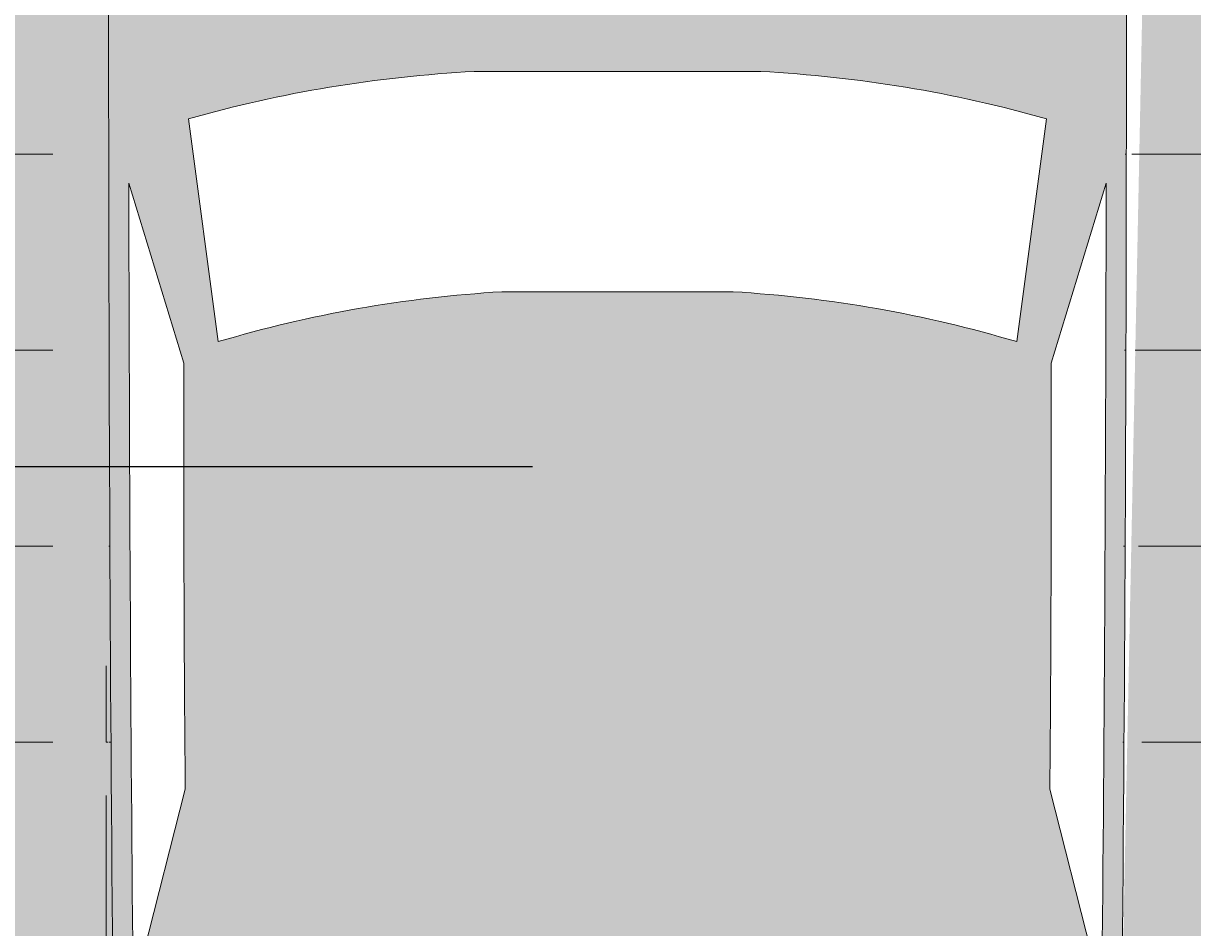
# Model space of a CAD drawing. Units: millimetres. Extents: x 1166 to 16630, y -7192 to 2820.
# Tile 4 of 8: x 5842 to 7051, y -4887 to -3952. Entities that reach past the tile are written whole.
import ezdxf

# ---------------------------------------------------------------- set-up
doc = ezdxf.new("R2010")
doc.units = ezdxf.units.MM
for name, color, linetype, lineweight in [('A-ANNO-DIMS', 2, 'Continuous', 18), ('A-FLOR-PATT', 8, 'Continuous', 13), ('C-PKNG-VEHI', 8, 'Continuous', 18)]:
    doc.layers.add(name, color=color, linetype=linetype, lineweight=lineweight)
doc.layers.add('A-FLOR-FNSH-PATT', color=254, linetype='Continuous', lineweight=13, true_color=0xfeeab9)
doc.layers.add('C-PKNG-VEHI-PATT', color=18, linetype='Continuous', lineweight=13, true_color=0x000000)
doc.styles.get("Standard").update_dxf_attribs({"font": 'arial.ttf'})
doc.dimstyles.get("Standard").update_dxf_attribs({"dimtxt": 0.18, "dimasz": 0.18, "dimexe": 0.18, "dimexo": 0.0625, "dimgap": 0.09, "dimtad": 0, "dimtih": 1, "dimtoh": 1, "dimdec": 4, "dimzin": 0, "dimdsep": 46, "dimtxsty": 'Standard', "dimcen": 0.09, "dimadec": 0, "dimazin": 0, "dimtfac": 1, "dimtdec": 4, "dimtofl": 0, "dimtmove": 0, "dimatfit": 3, "dimfxl": 1, "dimtolj": 1, "dimtzin": 0, "dimarcsym": 0})

# ---------------------------------------------------------------- blocks, each defined once
blk = doc.blocks.new('*U6')
for p, q in [((87.98532186932616, 31.87120872459877), (74.75900729854769, 35.92175679182955)), ((134.313356548143, 35.6043097713567), (119.2882629232503, 31.77757799177584)), ((70.0302824853563, 31.53613089391356), (86.40615155322342, 29.35124891408057)), ((66.55009204259746, -10.5288681329018), (66.55009204259746, 10.52886813290129)), ((82.73706193978568, 8.496039918672748), (82.73706193978568, -8.49603991867258)), ((86.40615155322318, -29.35124891408145), (70.03028248535594, -31.53613089391442)), ((134.3133565481428, -35.60430977135721), (119.2882629232503, -31.77757799177618)), ((87.98532186932607, -31.87120872459903), (74.7590072985476, -35.92175679182964))]:
    blk.add_line(p, q)
for centre, major_axis, ratio, start_param, end_param in [((64.48199294511879, -10555.61767587835), (1.907644e-10, 10593.02630634627), 0.842303869543847, -0.0133969486112073, 0.0027970409639888), ((64.4819929449925, -10555.61767590795), (1.9177683e-09, -10591.54646030096), 0.8423038695482963, 3.133765086725325, 3.140440689641252), ((95.78879860270445, -3666.353346297651), (1.949864e-10, -3698.236159209632), 0.8423038695446962, 3.134048706297306, 3.14409775411291), ((135.2911776514449, 5.387441675478555), (2.2715e-12, 81.77258453065997), 0.8423038695439563, 1.245306111696802, 1.507880129813836), ((149.595361812917, 2.799442537139299), (8.561e-13, -79.57966406425402), 0.842303869543983, 4.372215489277867, 4.640744122441986), ((149.5953618129329, -2.799442537137565), (4.0897e-12, -79.57966406427697), 0.8423038695439419, -1.499151468852248, -1.230622835688196), ((135.2911776514465, -5.387441675480715), (3.2038e-12, -81.77258453066244), 0.8423038695439492, -1.50788012981387, -1.245306111696839), ((95.78879860271888, 3666.35334629765), (1.637818e-10, -3698.236159209629), 0.8423038695447546, -0.0025051005232382, 0.007543947292366), ((64.48199294503607, 10555.61767590793), (1.6049794e-09, -10591.54646030094), 0.8423038695397146, 0.0011519639481523, 0.0078275668641468), ((64.48199294495228, 10555.61767590795), (6.117947e-10, 10593.02630637587), 0.8423038695458146, 3.138795612625926, 3.154989602201039)]:
    blk.add_ellipse(centre, major_axis=major_axis, ratio=ratio, start_param=start_param, end_param=end_param)
blk = doc.blocks.new('*D69')
at = {"layer": 'A-ANNO-DIMS', "color": 0, "lineweight": -2, "transparency": 16777216}
for p, q in [((2812.839545999997, -4410.708250999998), (2813.019545999998, -4410.708250999998)), ((2812.929545999998, -4410.798250999998), (2812.929545999998, -4410.618250999998)), ((6334.94458279999, -4410.707849399996), (5014.368944, -4410.707999979473))]:
    blk.add_line(p, q, dxfattribs=at)
at = {"layer": 'A-ANNO-DIMS', "color": 0, "transparency": 16777216}
blk.add_solid([(5014.36894399658, -4410.677999979474), (5014.368944003422, -4410.737999979473), (5014.188944, -4410.707999999998)], dxfattribs=at)
at = {"layer": 'Defpoints', "color": 0, "transparency": 16777216}
for p in [(2812.929545999998, -4410.708250999998), (5014.188944, -4410.707999999998)]:
    blk.add_point(p, dxfattribs=at)
at = {"layer": 'A-ANNO-DIMS', "color": 0, "transparency": 16777216, "insert": (6335.494344055106, -4410.707849399996), "char_height": 0.18, "attachment_point": 5}
blk.add_mtext('\\A1;R2201.3', dxfattribs=at)
blk = doc.blocks.new('*D70')
at = {"layer": 'A-ANNO-DIMS', "color": 0, "lineweight": -2, "transparency": 16777216}
for p, q in [((3047.988206, -4410.708432999997), (3048.168206000001, -4410.708432999997)), ((3048.078206, -4410.798432999997), (3048.078206, -4410.618432999997)), ((6368.217169199974, -4410.707740199998), (5123.345058, -4410.707999962437))]:
    blk.add_line(p, q, dxfattribs=at)
at = {"layer": 'A-ANNO-DIMS', "color": 0, "transparency": 16777216}
blk.add_solid([(5123.34505799374, -4410.677999962437), (5123.34505800626, -4410.737999962437), (5123.165058, -4410.707999999998)], dxfattribs=at)
at = {"layer": 'Defpoints', "color": 0, "transparency": 16777216}
for p in [(3048.078206, -4410.708432999998), (5123.165058, -4410.707999999998)]:
    blk.add_point(p, dxfattribs=at)
at = {"layer": 'A-ANNO-DIMS', "color": 0, "transparency": 16777216, "insert": (6368.662749008977, -4410.707740199998), "char_height": 0.18, "attachment_point": 5}
blk.add_mtext('\\A1;R2075', dxfattribs=at)

msp = doc.modelspace()

# ---------------------------------------------------------------- hatches: boundary and pattern name
at = {"layer": 'A-FLOR-FNSH-PATT', "transparency": 33554590}
h = msp.add_hatch(color=256, dxfattribs=at)
h.dxf.hatch_style = 1
h.paths.add_polyline_path([(5309.614992693758, -2642.53776490782), (5309.614992693758, -6304.141088113749), (7725.939441137629, -6304.141088113749), (7725.939441137629, -5672.53776490782), (7725.939441137629, -2642.53776490782)])
edge = h.paths.add_edge_path(flags=16)
edge.add_ellipse((-448.9724108440159, -3645.429588524165), major_axis=(-7430.722679011307, 2.05049e-10), ratio=0.8423038695440578, start_angle=182.1799503136468, end_angle=183.6504275857006, ccw=False)
edge.add_line((6974.17381326888, -3362.862478220109), (6984.715647929133, -3362.862478220109))
edge.add_ellipse((6982.28108362224, -3380.396843230207), major_axis=(-20.81714882728829, 5.19e-13), ratio=0.842303869543992, start_angle=180.0000000000014, end_angle=270.0000000000014, ccw=False)
edge.add_line((7003.098232449528, -3380.396843230198), (7003.098232449528, -3722.915565549822))
edge.add_ellipse((6982.28108362224, -3720.864922613471), major_axis=(20.81714882728829, 5.097e-13), ratio=0.842303869543992, start_angle=269.9999999999985, end_angle=359.9999999999986, ccw=False)
edge.add_ellipse((-142030.922985108, -3973.064272051784), major_axis=(149013.2040687302, 7.3876543e-09), ratio=0.8423038695454406, start_angle=-0.3838667787953227, end_angle=0.09022908859151357, ccw=False)
edge.add_line((6977.567346638728, -4971.397229994678), (6984.470063297348, -4971.397229994678))
edge.add_ellipse((6982.28108362224, -4988.931595004776), major_axis=(20.81714882728829, 5.4695e-12), ratio=0.84230386954397, start_angle=-1.5006662579253316e-11, end_angle=89.99999999998488, ccw=False)
edge.add_line((7003.098232449528, -4988.931595004766), (7003.098232449527, -5331.243460438734))
edge.add_ellipse((6982.281083622239, -5329.399674388036), major_axis=(-20.81714882728829, 1.0505e-12), ratio=0.84230386954397, start_angle=90.0000000000029, end_angle=180.000000000003, ccw=False)
edge.add_line((6982.281083622243, -5346.934039398132), (6973.353954790083, -5346.934039398132))
edge.add_ellipse((-142030.922985108, -3973.064272051784), major_axis=(149013.2040687302, 7.3876543e-09), ratio=0.8423038695454406, start_angle=-0.6186431963221253, end_angle=-0.5282714718208013, ccw=False)
edge.add_ellipse((6960.189207408767, -5606.902802775503), major_axis=(-31.22572324093233, 2.0889e-12), ratio=0.8423038695439425, start_angle=179.3717627838109, end_angle=248.4647566010108, ccw=False)
edge.add_ellipse((-142041.331559525, -3973.064272085929), major_axis=(-149045.3717863939, 4.64621177404e-05), ratio=0.8423038661083152, start_angle=179.3534459208122, end_angle=179.3717628016453, ccw=False)
edge.add_ellipse((6916.869834512962, -5654.054118847628), major_axis=(-73.80201542105252, 3.6097e-12), ratio=0.8423038695439748, start_angle=90.00000000006492, end_angle=179.353445902922, ccw=False)
edge.add_line((6916.869834513031, -5716.217842016925), (5995.230132669023, -5716.217842016909))
edge.add_ellipse((5995.230132669163, -5654.054118847574), major_axis=(73.80201542109666, 3.978e-13), ratio=0.8423038695439887, start_angle=180.6465540970575, end_angle=269.9999999998622, ccw=False)
edge.add_ellipse((154953.4315273228, -3973.06427200764), major_axis=(-149045.3717871212, 2.2898328512e-06), ratio=0.8423038697262194, start_angle=0.6282372171232851, end_angle=0.6465540979564253, ccw=False)
edge.add_ellipse((5951.910759773294, -5606.902802775455), major_axis=(31.22572324094488, 4.9039e-12), ratio=0.842303869543988, start_angle=111.53524350401449, end_angle=180.6282372161637, ccw=False)
edge.add_ellipse((154943.0229527065, -3973.064272049507), major_axis=(-149013.2040691466, 7.4869171e-09), ratio=0.8423038695459824, start_angle=0.528271471820176, end_angle=0.6465540970638131, ccw=False)
edge.add_line((5938.746012391977, -5346.934039398132), (5927.384319252956, -5346.934039398132))
edge.add_ellipse((5929.818883559845, -5329.399674388033), major_axis=(20.8171488272892, 3.11e-13), ratio=0.8423038695440205, start_angle=179.9999999999992, end_angle=269.9999999999962, ccw=False)
edge.add_line((5909.001734732555, -5329.399674388034), (5909.001734732554, -4986.88095206843))
edge.add_ellipse((5929.818883559843, -4988.931595004776), major_axis=(-20.8171488272892, 3.063e-13), ratio=0.8423038695440205, start_angle=-89.99999999999608, end_angle=7.958078640513122e-13, ccw=False)
edge.add_line((5929.818883559843, -4971.397229994676), (5934.53262054336, -4971.397229994676))
edge.add_ellipse((154943.0229527065, -3973.064272049507), major_axis=(-149013.2040691466, 7.4869171e-09), ratio=0.8423038695459824, start_angle=-0.09022908859031986, end_angle=0.38386677879520903, ccw=False)
edge.add_ellipse((5929.818883559843, -3720.864922613471), major_axis=(-20.8171488272892, 1.5867e-12), ratio=0.8423038695439331, start_angle=4.376943252282217e-12, end_angle=90.00000000000438, ccw=False)
edge.add_line((5909.001734732555, -3720.864922613478), (5909.001734732555, -3378.346200293855))
edge.add_ellipse((5929.818883559843, -3380.396843230207), major_axis=(20.8171488272892, 9.396e-13), ratio=0.8423038695439548, start_angle=89.99999999999739, end_angle=179.9999999999975, ccw=False)
edge.add_line((5929.818883559843, -3362.862478220109), (5937.926153913206, -3362.862478220109))
edge.add_ellipse((13361.0723780261, -3645.42958852417), major_axis=(7430.722679011307, 7.96527e-11), ratio=0.8423038695440075, start_angle=176.3495724143003, end_angle=177.8200496863542, ccw=False)
edge.add_ellipse((6843.238962592569, -6808.26137511002), major_axis=(4407.332901654202, 4.993684e-10), ratio=0.8423038695438785, start_angle=102.12596555227748, end_angle=103.7805289894913, ccw=False)
edge.add_ellipse((6843.238962592481, -6711.831352601092), major_axis=(4294.727564406183, 8.108409e-10), ratio=0.8423038695438188, start_angle=100.20953899713243, end_angle=102.4446272934332, ccw=False)
edge.add_ellipse((5718.978043047074, -189.3416182050969), major_axis=(-3530.283493235897, 2.29487e-11), ratio=0.8423038695439934, start_angle=99.25656600720184, end_angle=102.5549326441376)
edge.add_line((6369.842688727707, -3111.939026631001), (6452.046781461999, -3066.482546539763))
edge.add_ellipse((6456.049983591043, -3074.756545497792), major_axis=(-10.40857441364578, 1.5838e-12), ratio=0.8423038695437935, start_angle=270.0000000000206, end_angle=307.9331304598557, ccw=False)
edge.add_ellipse((6456.049983591043, -3074.756545497792), major_axis=(-10.40857441364578, 1.5838e-12), ratio=0.8423038695437935, start_angle=232.06686954016618, end_angle=270.0000000000206, ccw=False)
edge.add_line((6461.762224667734, -3067.427595530816), (6542.257278454378, -3111.939026631002))
edge.add_ellipse((7193.121924135012, -189.3416182050969), major_axis=(3530.283493235459, 5.426614e-10), ratio=0.842303869544094, start_angle=257.4450673558539, end_angle=260.7434339927895)
edge.add_ellipse((6068.861004589511, -6711.831352601148), major_axis=(4294.72756440461, 7.517164e-10), ratio=0.8423038695441345, start_angle=77.55537270654469, end_angle=79.79046100284552, ccw=False)
edge.add_ellipse((6068.86100458951, -6808.26137511002), major_axis=(-4407.332901654327, 6.637773e-10), ratio=0.842303869543856, start_angle=256.2194710105107, end_angle=257.8740344477245, ccw=False)
edge = h.paths.add_edge_path(flags=0)
edge.add_ellipse((5799.636342679871, -3484.80630294614), major_axis=(790.1331889300527, 2.1537e-12), ratio=0.8423038695439757, start_angle=-2.2737367544323206e-13, end_angle=29.43856959797921, ccw=False)
edge.add_line((6589.769531609924, -3484.806302946152), (6589.769531609924, -3517.865771969153))
edge.add_line((6589.769531609924, -3517.865771969153), (6615.396946753699, -3517.865771969153))
edge.add_ellipse((6612.950235160742, -3526.632954474201), major_axis=(10.40857441364348, 1.5653e-12), ratio=0.8423038695440233, start_angle=45.51978911742219, end_angle=89.99999999999147, ccw=False)
edge.add_line((6619.58436781158, -3519.877346340421), (6697.576744801804, -3574.216072032502))
edge.add_line((6697.576744801804, -3574.216072032502), (6697.576744801804, -3782.552340767745))
edge.add_ellipse((6643.673138205864, -3780.461483581003), major_axis=(5.016450041930374, 89.18653102701357), ratio=0.6038335755719256, start_angle=106.34259195429391, end_angle=270.99798572497, ccw=False)
edge.add_line((6589.769531609924, -3793.028339937766), (6589.769531609924, -3484.806302946153))
edge.add_ellipse((5799.636342679871, -3484.80630294614), major_axis=(790.1331889300527, 2.1537e-12), ratio=0.8423038695439757, start_angle=-2.143e-13, end_angle=29.43856959797918)
edge.add_ellipse((7112.463624502211, -3484.80630294614), major_axis=(-790.1331889300524, 7.9434e-12), ratio=0.8423038695439707, start_angle=-29.43856959797882, end_angle=5.465e-13)
edge.add_line((6322.330435572158, -3484.806302946151), (6322.330435572158, -3793.028339937766))
edge.add_ellipse((6268.426828976219, -3780.461483581003), major_axis=(-5.016450041930374, 89.18653102701357), ratio=0.6038335755719256, start_angle=89.00201427502998, end_angle=253.6574080457062, ccw=False)
edge.add_line((6214.523222380278, -3782.552340767737), (6214.523222380279, -3574.216072032502))
edge.add_line((6214.523222380279, -3574.216072032502), (6294.400928520307, -3518.563802793423))
edge.add_ellipse((6299.149732021341, -3526.632954474201), major_axis=(10.4085744136453, 3.381e-13), ratio=0.8423038695438764, start_angle=89.9999999999983, end_angle=134.4802108825654, ccw=False)
edge.add_line((6299.149732021338, -3517.865771969152), (6322.330435572158, -3517.865771969152))
edge.add_line((6322.330435572158, -3517.865771969152), (6322.330435572158, -3484.806302946154))
edge.add_ellipse((7112.463624502211, -3484.80630294614), major_axis=(-790.1331889300524, 7.9434e-12), ratio=0.8423038695439707, start_angle=-29.438569597978812, end_angle=6.252776074688882e-13, ccw=False)
edge = h.paths.add_edge_path(flags=0)
edge.add_line((6899.672020630411, -4051.112638739672), (6868.937058315451, -4281.473694083312))
edge.add_ellipse((6495.430033257824, -5170.362894493258), major_axis=(1119.455420763322, 3.0514e-12), ratio=0.8423038695439744, start_angle=67.20808512240981, end_angle=85.12993040286408)
edge.add_line((6575.564661792019, -4229.860228440724), (6336.53530539007, -4229.860228440724))
edge.add_ellipse((6416.669933924288, -5170.362894493482), major_axis=(1119.455420763633, 5.82337e-11), ratio=0.842303869543943, start_angle=94.87006959713275, end_angle=112.7919148775836)
edge.add_line((6043.162908866626, -4281.473694083309), (6012.427946551666, -4051.112638739666))
edge.add_ellipse((6380.264280565288, -4969.144446445703), major_axis=(1150.303461305961, 5.9583e-11), ratio=0.8423038695439412, start_angle=94.27742096305099, end_angle=111.83495379670521, ccw=False)
edge.add_line((6307.939299228742, -4002.156437400477), (6604.160667953341, -4002.156437400477))
edge.add_ellipse((6531.835686616772, -4969.144446445682), major_axis=(-1150.303461305901, 2.25473e-11), ratio=0.8423038695439672, start_angle=248.1650462032914, end_angle=265.72257903694555, ccw=False)
edge = h.paths.add_edge_path(flags=0)
edge.add_ellipse((-142030.9229855244, -3973.064272050007), major_axis=(-148992.3869203194, 2.076209e-10), ratio=0.842303869544003, start_angle=179.6222358060902, end_angle=179.9444056865007, ccw=False)
edge.add_line((6956.899516505626, -4955.389335168179), (6903.06848209712, -4744.029778632651))
edge.add_ellipse((-45118.92430422086, -4413.460367112857), major_axis=(52023.47313689829, 7.771381e-10), ratio=0.842303869543516, start_angle=-0.3640763488911976, end_angle=0.1208973690317991)
edge.add_line((6904.3855953652, -4303.688047353878), (6961.365076797346, -4117.63210307358))
edge = h.paths.add_edge_path(flags=0)
edge.add_line((5950.734890384741, -4117.632103073563), (6007.714371816899, -4303.688047353918))
edge.add_ellipse((58031.02427140294, -4413.460367113082), major_axis=(-52023.47313689826, 1.3200601e-09), ratio=0.8423038695497072, start_angle=-0.1208973690315197, end_angle=0.364076348891516)
edge.add_line((6009.031485084967, -4744.029778632643), (5955.200450676423, -4955.389335168309))
edge.add_ellipse((154943.0229527063, -3973.064272050686), major_axis=(-148992.3869203192, 3.28274152e-08), ratio=0.8423038695536886, start_angle=0.05559431351167632, end_angle=0.3777641939223031, ccw=False)
edge = h.paths.add_edge_path(flags=0)
edge.add_line((6868.937058315452, -5013.198477251068), (6868.937058315452, -5277.993200767081))
edge.add_ellipse((6456.049983591043, -3571.079447459644), major_axis=(2068.11644385622, 7.9333e-12), ratio=0.8423038695439821, start_angle=256.4018653097692, end_angle=283.59813469023027, ccw=False)
edge.add_line((6043.16290886663, -5277.993200767081), (6043.16290886663, -5013.198477251068))
edge.add_ellipse((6456.049983591043, -3306.284723943631), major_axis=(2068.116443856253, 3.3411e-12), ratio=0.8423038695439679, start_angle=256.4018653097692, end_angle=283.5981346902304)
edge = h.paths.add_edge_path(flags=0)
edge.add_ellipse((6827.302760660877, -5415.313265203762), major_axis=(-41.63429765457658, 1.038e-12), ratio=0.842303869543992, start_angle=180.0000000000014, end_angle=270.0000000000014, ccw=False)
edge.add_line((6868.937058315454, -5415.313265203762), (6868.937058315454, -5689.12284886784))
edge.add_line((6868.937058315454, -5689.12284886784), (6043.162908866631, -5689.122848867824))
edge.add_line((6043.162908866631, -5689.122848867824), (6043.16290886663, -5415.313265203758))
edge.add_ellipse((6084.797206521206, -5415.313265203759), major_axis=(-41.63429765457658, 3.4138e-12), ratio=0.842303869543992, start_angle=-89.99999999999523, end_angle=4.718003765447065e-12, ccw=False)
edge.add_line((6084.797206521207, -5380.244535183563), (6827.302760660879, -5380.244535183566))
h.paths.add_polyline_path([(3455.939441137629, -522.53776490782), (1955.939441137629, -522.53776490782), (1955.939441137629, -2522.53776490782), (3455.939441137629, -2522.53776490782), (3455.939441137628, -2456.640093510054), (2713.439441137629, -2456.640093510054), (2713.43944113763, -2423.827593510054), (2714.157558370035, -2423.827593510054, -0.398552660000795), (3455.939441137629, -1706.6775944476)])
h.paths.add_polyline_path([(2617.666699633915, -1084.404517764245, -0.1328909081885223), (2584.2707950462, -1084.404517500826, -0.5013167773008519), (2505.064916213601, -782.9330743979599), (2537.033121160981, -687.0284595558127), (2489.081652205778, -687.0284595558132), (2489.081652205778, -711.0041940334158), (2441.130183250573, -711.0041940334158), (2441.130183250573, -695.0203710483474), (2473.097829220709, -695.0203710483474), (2473.097829220709, -687.0284595558132), (2433.13827175804, -687.0284595558132), (2433.138271758038, -559.1578756752674), (2768.79855444447, -559.1578756752674), (2768.798554444471, -687.0284595558132), (2664.903705041528, -687.0284595558132), (2696.870765296628, -782.9296403211174, -0.5013234908365807)], flags=16)
h.paths.add_polyline_path([(2627.246667254758, -1063.015793855155, -0.2150037826753064), (2574.690827957319, -1063.015793301825, -0.4800796505537303), (2537.033991046725, -782.9313974662227), (2664.904416594217, -782.9313974662227, -0.4800795019660876)], flags=0)
h.paths.add_polyline_path([(2736.830905816404, -671.0446365707452), (2465.105920386107, -671.0446365707452, -0.5000001164022092), (2449.122094743107, -655.0608109277463), (2449.122094743107, -591.1255243033341, -0.5000001164022404), (2465.105920386111, -575.1416986603361), (2736.830905816402, -575.1416986603361, -0.5000001164023353), (2752.814731459403, -591.1255243033406), (2752.814731459403, -655.0608109277468, -0.50000011640211)], flags=0)
h.paths.add_polyline_path([(5931.781743219382, -6111.826019846759), (7070.309755611069, -6111.826019846759), (7070.309755611069, -5852.301891921869), (5931.781743219382, -5852.301891921869)], flags=24)
h.paths.add_polyline_path([(2102.335631979146, -1543.656328414819), (3007.075088498303, -1543.656328414819), (3007.075088498303, -1283.961010431932), (2102.335631979146, -1283.961010431932)], flags=24)
at = {"layer": 'A-FLOR-PATT', "transparency": 33554564}
h = msp.add_hatch(dxfattribs=at)
h.set_pattern_fill('ANGLE', color=256, scale=29)
h.set_pattern_definition([(0, (-8657.519420588213, -11987.85165359825), (0, 202.565), [147.32, -55.24499999999999]), (90, (-8657.519420588213, -11987.85165359825), (-202.565, 1.24e-14), [147.32, -55.24499999999999])])
h.paths.add_polyline_path([(7725.939441137629, -2642.53776490782), (5309.614992693758, -2642.53776490782), (5309.614992693758, -6304.141088113749), (7725.939441137629, -6304.141088113749), (7725.939441137629, -5672.53776490782)])
edge = h.paths.add_edge_path(flags=16)
edge.add_ellipse((-142030.922985108, -3973.064272051784), major_axis=(149013.2040687302, 7.3876543e-09), ratio=0.8423038695454406, start_angle=-0.3838667787953227, end_angle=0.09022908859151357, ccw=False)
edge.add_ellipse((6982.28108362224, -4988.931595004776), major_axis=(20.81714882728829, 5.4695e-12), ratio=0.84230386954397, start_angle=-1.5006662579253316e-11, end_angle=89.99999999998488, ccw=False)
edge.add_line((7003.098232449528, -4988.931595004773), (7003.098232449527, -5329.399674388036))
edge.add_ellipse((6982.281083622239, -5329.399674388036), major_axis=(-20.81714882728829, 1.0505e-12), ratio=0.84230386954397, start_angle=90.0000000000029, end_angle=180.000000000003, ccw=False)
edge.add_line((6982.281083622241, -5346.934039398132), (6973.353954790083, -5346.934039398132))
edge.add_ellipse((-142030.922985108, -3973.064272051784), major_axis=(149013.2040687302, 7.3876543e-09), ratio=0.8423038695454406, start_angle=-0.6186431963221253, end_angle=-0.5282714718208013, ccw=False)
edge.add_ellipse((6960.189207408767, -5606.902802775503), major_axis=(-31.22572324093233, 2.0889e-12), ratio=0.8423038695439425, start_angle=179.3717627838109, end_angle=248.4647566010108, ccw=False)
edge.add_ellipse((-142041.331559525, -3973.064272085929), major_axis=(-149045.3717863939, 4.64621177404e-05), ratio=0.8423038661083152, start_angle=179.3534459208122, end_angle=179.3717628016453, ccw=False)
edge.add_ellipse((6916.869834512962, -5654.054118847628), major_axis=(-73.80201542105252, 3.6097e-12), ratio=0.8423038695439748, start_angle=90.00000000006492, end_angle=179.353445902922, ccw=False)
edge.add_line((6916.869834513029, -5716.217842016925), (5995.230132669016, -5716.217842016909))
edge.add_ellipse((5995.230132669163, -5654.054118847574), major_axis=(73.80201542109666, 3.978e-13), ratio=0.8423038695439887, start_angle=180.6465540970575, end_angle=269.9999999998622, ccw=False)
edge.add_ellipse((154953.4315273228, -3973.06427200764), major_axis=(-149045.3717871212, 2.2898328512e-06), ratio=0.8423038697262194, start_angle=0.6282372171232851, end_angle=0.6465540979564253, ccw=False)
edge.add_ellipse((5951.910759773294, -5606.902802775455), major_axis=(31.22572324094488, 4.9039e-12), ratio=0.842303869543988, start_angle=111.53524350401449, end_angle=180.6282372161637, ccw=False)
edge.add_ellipse((154943.0229527065, -3973.064272049507), major_axis=(-149013.2040691466, 7.4869171e-09), ratio=0.8423038695459824, start_angle=0.528271471820176, end_angle=0.6465540970638131, ccw=False)
edge.add_line((5938.746012391977, -5346.934039398132), (5929.818883559843, -5346.934039398132))
edge.add_ellipse((5929.818883559845, -5329.399674388033), major_axis=(20.8171488272892, 3.11e-13), ratio=0.8423038695440205, start_angle=179.9999999999992, end_angle=269.9999999999962, ccw=False)
edge.add_line((5909.001734732555, -5329.399674388033), (5909.001734732554, -4988.931595004778))
edge.add_ellipse((5929.818883559843, -4988.931595004776), major_axis=(-20.8171488272892, 3.063e-13), ratio=0.8423038695440205, start_angle=-89.99999999999608, end_angle=7.958078640513122e-13, ccw=False)
edge.add_ellipse((154943.0229527065, -3973.064272049507), major_axis=(-149013.2040691466, 7.4869171e-09), ratio=0.8423038695459824, start_angle=-0.09022908859031986, end_angle=0.38386677879520903, ccw=False)
edge.add_ellipse((5929.818883559843, -3720.864922613471), major_axis=(-20.8171488272892, 1.5867e-12), ratio=0.8423038695439331, start_angle=4.376943252282217e-12, end_angle=90.00000000000438, ccw=False)
edge.add_line((5909.001734732555, -3720.864922613472), (5909.001734732555, -3380.396843230204))
edge.add_ellipse((5929.818883559843, -3380.396843230207), major_axis=(20.8171488272892, 9.396e-13), ratio=0.8423038695439548, start_angle=89.99999999999739, end_angle=179.9999999999975, ccw=False)
edge.add_line((5929.818883559843, -3362.862478220109), (5937.926153913207, -3362.862478220109))
edge.add_ellipse((13361.0723780261, -3645.42958852417), major_axis=(7430.722679011307, 7.96527e-11), ratio=0.8423038695440075, start_angle=176.3495724143003, end_angle=177.8200496863542, ccw=False)
edge.add_ellipse((6843.238962592569, -6808.26137511002), major_axis=(4407.332901654202, 4.993684e-10), ratio=0.8423038695438785, start_angle=102.12596555227748, end_angle=103.7805289894913, ccw=False)
edge.add_ellipse((6843.238962592481, -6711.831352601092), major_axis=(4294.727564406183, 8.108409e-10), ratio=0.8423038695438188, start_angle=100.20953899713243, end_angle=102.4446272934332, ccw=False)
edge.add_ellipse((5718.978043047074, -189.3416182050969), major_axis=(-3530.283493235897, 2.29487e-11), ratio=0.8423038695439934, start_angle=99.25656600720184, end_angle=102.5549326441376)
edge.add_line((6369.842688727707, -3111.939026631), (6453.505541262713, -3065.675894661087))
edge.add_ellipse((6456.049983591043, -3074.756545497792), major_axis=(-10.40857441364578, 1.5838e-12), ratio=0.8423038695437935, start_angle=232.06686954016618, end_angle=270.0000000000206, ccw=False)
edge.add_line((6460.053185720086, -3066.482546539763), (6542.257278454378, -3111.939026631002))
edge.add_ellipse((7193.121924135012, -189.3416182050969), major_axis=(3530.283493235459, 5.426614e-10), ratio=0.842303869544094, start_angle=257.4450673558539, end_angle=260.7434339927895)
edge.add_ellipse((6068.861004589511, -6711.831352601148), major_axis=(4294.72756440461, 7.517164e-10), ratio=0.8423038695441345, start_angle=77.55537270654469, end_angle=79.79046100284552, ccw=False)
edge.add_ellipse((6068.86100458951, -6808.26137511002), major_axis=(-4407.332901654327, 6.637773e-10), ratio=0.842303869543856, start_angle=256.2194710105107, end_angle=257.8740344477245, ccw=False)
edge.add_ellipse((-448.9724108440159, -3645.429588524165), major_axis=(-7430.722679011307, 2.05049e-10), ratio=0.8423038695440578, start_angle=182.1799503136468, end_angle=183.6504275857006, ccw=False)
edge.add_line((6974.17381326888, -3362.862478220109), (6982.28108362224, -3362.862478220109))
edge.add_ellipse((6982.28108362224, -3380.396843230207), major_axis=(-20.81714882728829, 5.19e-13), ratio=0.842303869543992, start_angle=180.0000000000014, end_angle=270.0000000000014, ccw=False)
edge.add_line((7003.098232449528, -3380.396843230204), (7003.098232449528, -3720.864922613474))
edge.add_ellipse((6982.28108362224, -3720.864922613471), major_axis=(20.81714882728829, 5.097e-13), ratio=0.842303869543992, start_angle=269.9999999999985, end_angle=359.9999999999986, ccw=False)
edge = h.paths.add_edge_path(flags=0)
edge.add_ellipse((-142030.9229855244, -3973.064272050007), major_axis=(-148992.3869203194, 2.076209e-10), ratio=0.842303869544003, start_angle=179.6222358060902, end_angle=179.9444056865007, ccw=False)
edge.add_line((6956.899516505626, -4955.389335168179), (6903.06848209712, -4744.029778632651))
edge.add_ellipse((-45118.92430422086, -4413.460367112857), major_axis=(52023.47313689829, 7.771381e-10), ratio=0.842303869543516, start_angle=-0.3640763488911976, end_angle=0.1208973690317991)
edge.add_line((6904.3855953652, -4303.688047353878), (6961.365076797346, -4117.632103073563))
edge = h.paths.add_edge_path(flags=0)
edge.add_line((6899.672020630411, -4051.112638739673), (6868.937058315451, -4281.473694083312))
edge.add_ellipse((6495.430033257824, -5170.362894493258), major_axis=(1119.455420763322, 3.0514e-12), ratio=0.8423038695439744, start_angle=67.20808512240981, end_angle=85.12993040286408)
edge.add_line((6575.564661792022, -4229.860228440724), (6336.535305390071, -4229.860228440724))
edge.add_ellipse((6416.669933924288, -5170.362894493482), major_axis=(1119.455420763633, 5.82337e-11), ratio=0.842303869543943, start_angle=94.87006959713275, end_angle=112.7919148775836)
edge.add_line((6043.162908866626, -4281.473694083308), (6012.427946551666, -4051.112638739666))
edge.add_ellipse((6380.264280565288, -4969.144446445703), major_axis=(1150.303461305961, 5.9583e-11), ratio=0.8423038695439412, start_angle=94.27742096305099, end_angle=111.83495379670521, ccw=False)
edge.add_line((6307.939299228742, -4002.156437400477), (6604.16066795334, -4002.156437400477))
edge.add_ellipse((6531.835686616772, -4969.144446445682), major_axis=(-1150.303461305901, 2.25473e-11), ratio=0.8423038695439672, start_angle=248.1650462032914, end_angle=265.72257903694555, ccw=False)
edge = h.paths.add_edge_path(flags=0)
edge.add_ellipse((6643.673138205864, -3780.461483581003), major_axis=(5.016450041930374, 89.18653102701357), ratio=0.6038335755719256, start_angle=106.34259195429391, end_angle=270.99798572497, ccw=False)
edge.add_line((6589.769531609924, -3793.028339937766), (6589.769531609924, -3484.806302946154))
edge.add_ellipse((5799.636342679871, -3484.80630294614), major_axis=(790.1331889300527, 2.1537e-12), ratio=0.8423038695439757, start_angle=-2.143e-13, end_angle=29.43856959797918)
edge.add_ellipse((7112.463624502211, -3484.80630294614), major_axis=(-790.1331889300524, 7.9434e-12), ratio=0.8423038695439707, start_angle=-29.43856959797882, end_angle=5.465e-13)
edge.add_line((6322.330435572158, -3484.806302946151), (6322.330435572158, -3793.028339937766))
edge.add_ellipse((6268.426828976219, -3780.461483581003), major_axis=(-5.016450041930374, 89.18653102701357), ratio=0.6038335755719256, start_angle=89.00201427502998, end_angle=253.6574080457062, ccw=False)
edge.add_line((6214.523222380278, -3782.552340767735), (6214.523222380279, -3574.216072032502))
edge.add_line((6214.523222380279, -3574.216072032502), (6295.402812213822, -3517.865771969152))
edge.add_line((6295.402812213822, -3517.865771969152), (6322.330435572158, -3517.865771969152))
edge.add_line((6322.330435572158, -3517.865771969152), (6322.330435572158, -3484.806302946154))
edge.add_ellipse((7112.463624502211, -3484.80630294614), major_axis=(-790.1331889300524, 7.9434e-12), ratio=0.8423038695439707, start_angle=-29.438569597978812, end_angle=6.252776074688882e-13, ccw=False)
edge.add_ellipse((5799.636342679871, -3484.80630294614), major_axis=(790.1331889300527, 2.1537e-12), ratio=0.8423038695439757, start_angle=-2.2737367544323206e-13, end_angle=29.43856959797921, ccw=False)
edge.add_line((6589.769531609924, -3484.806302946153), (6589.769531609924, -3517.865771969153))
edge.add_line((6589.769531609924, -3517.865771969153), (6616.697154968261, -3517.865771969153))
edge.add_line((6616.697154968261, -3517.865771969153), (6697.576744801804, -3574.216072032502))
edge.add_line((6697.576744801804, -3574.216072032502), (6697.576744801804, -3782.552340767746))
edge = h.paths.add_edge_path(flags=0)
edge.add_line((6868.937058315452, -5013.198477251068), (6868.937058315452, -5277.993200767081))
edge.add_ellipse((6456.049983591043, -3571.079447459644), major_axis=(2068.11644385622, 7.9333e-12), ratio=0.8423038695439821, start_angle=256.4018653097692, end_angle=283.59813469023027, ccw=False)
edge.add_line((6043.16290886663, -5277.993200767081), (6043.16290886663, -5013.198477251067))
edge.add_ellipse((6456.049983591043, -3306.284723943631), major_axis=(2068.116443856253, 3.3411e-12), ratio=0.8423038695439679, start_angle=256.4018653097692, end_angle=283.5981346902304)
edge = h.paths.add_edge_path(flags=0)
edge.add_ellipse((58031.02427140294, -4413.460367113082), major_axis=(-52023.47313689826, 1.3200601e-09), ratio=0.8423038695497072, start_angle=-0.1208973690315197, end_angle=0.364076348891516)
edge.add_line((6009.031485084967, -4744.029778632643), (5955.200450676423, -4955.389335168309))
edge.add_ellipse((154943.0229527063, -3973.064272050686), major_axis=(-148992.3869203192, 3.28274152e-08), ratio=0.8423038695536886, start_angle=0.05559431351167632, end_angle=0.3777641939223031, ccw=False)
edge.add_line((5950.734890384742, -4117.632103073569), (6007.714371816899, -4303.688047353918))
edge = h.paths.add_edge_path(flags=0)
edge.add_ellipse((6827.302760660877, -5415.313265203762), major_axis=(-41.63429765457658, 1.038e-12), ratio=0.842303869543992, start_angle=180.0000000000014, end_angle=270.0000000000014, ccw=False)
edge.add_line((6868.937058315454, -5415.313265203762), (6868.937058315454, -5689.12284886784))
edge.add_line((6868.937058315454, -5689.12284886784), (6043.162908866631, -5689.122848867824))
edge.add_line((6043.162908866631, -5689.122848867824), (6043.16290886663, -5415.31326520376))
edge.add_ellipse((6084.797206521206, -5415.313265203759), major_axis=(-41.63429765457658, 3.4138e-12), ratio=0.842303869543992, start_angle=-89.99999999999523, end_angle=4.718003765447065e-12, ccw=False)
edge.add_line((6084.797206521206, -5380.244535183563), (6827.302760660877, -5380.244535183566))
at = {"layer": 'C-PKNG-VEHI-PATT'}
h = msp.add_hatch(color=256, dxfattribs=at)
h.dxf.hatch_style = 1
edge = h.paths.add_edge_path()
edge.add_ellipse((-142030.922985108, -3973.064272051784), major_axis=(149013.2040687302, 7.3876543e-09), ratio=0.8423038695454406, start_angle=-0.3838667787953527, end_angle=0.0902290885914815)
edge.add_ellipse((-142030.922985108, -3973.064272051784), major_axis=(149013.2040687302, 7.3876543e-09), ratio=0.8423038695454406, start_angle=0.0902290885914815, end_angle=0.1349865768554186)
edge.add_ellipse((-448.9724108440159, -3645.429588524165), major_axis=(-7430.722679011307, 2.05049e-10), ratio=0.8423038695440578, start_angle=180.1356123904399, end_angle=182.1799503136467)
edge.add_ellipse((-448.9724108440159, -3645.429588524165), major_axis=(-7430.722679011307, 2.05049e-10), ratio=0.8423038695440578, start_angle=182.1799503136467, end_angle=183.6504275857006)
edge.add_ellipse((6068.86100458951, -6808.26137511002), major_axis=(-4407.332901654327, 6.637773e-10), ratio=0.842303869543856, start_angle=256.2194710105107, end_angle=257.8740344477245)
edge.add_ellipse((-1899.27789287437, -3593.136558560746), major_axis=(-8768.422834748915, 4.33705e-11), ratio=0.8423038695439387, start_angle=177.8014594340451, end_angle=182.8637146078378, ccw=False)
edge.add_ellipse((6531.835686616759, -4956.613487829934), major_axis=(1262.90879855413, 2.05481e-11), ratio=0.8423038695439913, start_angle=72.28004677724863, end_angle=85.91758930884843)
edge.add_line((6607.621389642485, -3894.777567489213), (6304.478577539601, -3894.777567489213))
edge.add_ellipse((6380.264280565318, -4956.613487829931), major_axis=(1262.908798554214, 5.95268e-11), ratio=0.8423038695439325, start_angle=94.08241069114744, end_angle=107.7199532227473)
edge.add_ellipse((14811.37786005643, -3593.136558560761), major_axis=(8768.422834748895, 2.19537e-11), ratio=0.8423038695438954, start_angle=177.1362853921622, end_angle=182.1985405659549, ccw=False)
edge.add_ellipse((6843.238962592569, -6808.26137511002), major_axis=(4407.332901654202, 4.993684e-10), ratio=0.8423038695438785, start_angle=102.1259655522775, end_angle=103.7805289894913)
edge.add_ellipse((13361.0723780261, -3645.42958852417), major_axis=(7430.722679011307, 7.96527e-11), ratio=0.8423038695440075, start_angle=176.3495724143003, end_angle=177.8200496863541)
edge.add_ellipse((13361.0723780261, -3645.42958852417), major_axis=(7430.722679011307, 7.96527e-11), ratio=0.8423038695440075, start_angle=177.8200496863541, end_angle=179.8643876095608)
edge.add_ellipse((154943.0229527065, -3973.064272049507), major_axis=(-149013.2040691466, 7.4869171e-09), ratio=0.8423038695459824, start_angle=-0.1349865768541338, end_angle=-0.0902290885903158)
edge.add_ellipse((154943.0229527065, -3973.064272049507), major_axis=(-149013.2040691466, 7.4869171e-09), ratio=0.8423038695459824, start_angle=-0.0902290885903158, end_angle=0.3838667787951928)
edge.add_ellipse((154943.0229527065, -3973.064272049507), major_axis=(-149013.2040691466, 7.4869171e-09), ratio=0.8423038695459824, start_angle=0.3838667787951928, end_angle=0.5282714718202328)
edge.add_ellipse((154943.0229527065, -3973.064272049507), major_axis=(-149013.2040691466, 7.4869171e-09), ratio=0.8423038695459824, start_angle=0.5282714718202328, end_angle=0.6465540970638061)
edge.add_ellipse((5984.821558255466, -5654.054118847628), major_axis=(41.63429765457481, 1.0657e-12), ratio=0.8423038695440057, start_angle=180.6465540970899, end_angle=269.9999999999108)
edge.add_line((5984.821558255388, -5689.122848867822), (6043.162908866631, -5689.122848867825))
edge.add_line((6043.162908866631, -5689.122848867825), (6043.16290886663, -5411.211979331063))
edge.add_ellipse((6084.797206521206, -5415.313265203759), major_axis=(-41.63429765457658, 3.4138e-12), ratio=0.842303869543992, start_angle=-89.99999999999523, end_angle=4.718003765447065e-12, ccw=False)
edge.add_line((6084.797206521205, -5380.244535183563), (6832.171889274661, -5380.244535183566))
edge.add_ellipse((6827.302760660877, -5415.313265203762), major_axis=(-41.63429765457658, 1.038e-12), ratio=0.842303869543992, start_angle=180.0000000000014, end_angle=270.0000000000014, ccw=False)
edge.add_line((6868.937058315454, -5415.313265203762), (6868.937058315454, -5689.12284886784))
edge.add_line((6868.937058315454, -5689.12284886784), (6927.278408926672, -5689.122848867841))
edge.add_ellipse((6927.278408926624, -5654.054118847645), major_axis=(-41.63429765457638, 9.732e-13), ratio=0.8423038695439738, start_angle=90.00000000008009, end_angle=179.3534459029312)
edge.add_ellipse((-142030.922985108, -3973.064272051784), major_axis=(149013.2040687302, 7.3876543e-09), ratio=0.8423038695454406, start_angle=-0.646554097064762, end_angle=-0.6186431963220466)
edge.add_ellipse((-142030.922985108, -3973.064272051784), major_axis=(149013.2040687302, 7.3876543e-09), ratio=0.8423038695454406, start_angle=-0.6186431963220466, end_angle=-0.5282714718207955)
edge.add_ellipse((-142030.922985108, -3973.064272051784), major_axis=(149013.2040687302, 7.3876543e-09), ratio=0.8423038695454406, start_angle=-0.5282714718207955, end_angle=-0.3838667787953527)
edge = h.paths.add_edge_path(flags=16)
edge.add_ellipse((6416.669933924288, -5170.362894493482), major_axis=(1119.455420763633, 5.82337e-11), ratio=0.842303869543943, start_angle=94.87006959713275, end_angle=112.7919148775836)
edge.add_line((6043.162908866626, -4281.473694083309), (6012.427946551666, -4051.112638739666))
edge.add_ellipse((6380.264280565288, -4969.144446445703), major_axis=(1150.303461305961, 5.9583e-11), ratio=0.8423038695439412, start_angle=94.27742096305099, end_angle=111.83495379670521, ccw=False)
edge.add_line((6307.93929922874, -4002.156437400477), (6604.16066795334, -4002.156437400477))
edge.add_ellipse((6531.835686616772, -4969.144446445682), major_axis=(-1150.303461305901, 2.25473e-11), ratio=0.8423038695439672, start_angle=248.1650462032914, end_angle=265.72257903694555, ccw=False)
edge.add_line((6899.672020630411, -4051.112638739672), (6868.937058315451, -4281.473694083312))
edge.add_ellipse((6495.430033257824, -5170.362894493258), major_axis=(1119.455420763322, 3.0514e-12), ratio=0.8423038695439744, start_angle=67.20808512240981, end_angle=85.12993040286408)
edge.add_line((6575.564661792022, -4229.860228440724), (6336.535305390071, -4229.860228440724))
edge = h.paths.add_edge_path(flags=16)
edge.add_ellipse((58031.02427140294, -4413.460367113082), major_axis=(-52023.47313689826, 1.3200601e-09), ratio=0.8423038695497072, start_angle=-0.1208973690315197, end_angle=0.364076348891516)
edge.add_line((6009.031485084967, -4744.029778632643), (5955.200450676423, -4955.389335168309))
edge.add_ellipse((154943.0229527063, -3973.064272050686), major_axis=(-148992.3869203192, 3.28274152e-08), ratio=0.8423038695536886, start_angle=0.05559431351167632, end_angle=0.3777641939223031, ccw=False)
edge.add_line((5950.734890384742, -4117.632103073569), (6007.714371816899, -4303.688047353918))
edge = h.paths.add_edge_path(flags=16)
edge.add_line((6904.3855953652, -4303.688047353878), (6961.365076797346, -4117.63210307357))
edge.add_ellipse((-142030.9229855244, -3973.064272050007), major_axis=(-148992.3869203194, 2.076209e-10), ratio=0.842303869544003, start_angle=179.6222358060902, end_angle=179.9444056865007, ccw=False)
edge.add_line((6956.899516505626, -4955.38933516818), (6903.06848209712, -4744.029778632651))
edge.add_ellipse((-45118.92430422086, -4413.460367112857), major_axis=(52023.47313689829, 7.771381e-10), ratio=0.842303869543516, start_angle=-0.3640763488911976, end_angle=0.1208973690317991)
edge = h.paths.add_edge_path(flags=16)
edge.add_ellipse((6456.049983591043, -3306.284723943631), major_axis=(2068.116443856253, 3.3411e-12), ratio=0.8423038695439679, start_angle=256.4018653097692, end_angle=283.5981346902304)
edge.add_line((6868.937058315452, -5013.198477251068), (6868.937058315452, -5277.993200767081))
edge.add_ellipse((6456.049983591043, -3571.079447459644), major_axis=(2068.11644385622, 7.9333e-12), ratio=0.8423038695439821, start_angle=256.4018653097692, end_angle=283.59813469023027, ccw=False)
edge.add_line((6043.16290886663, -5277.993200767081), (6043.16290886663, -5013.198477251067))

# ---------------------------------------------------------------- block references
at = {"layer": 'C-PKNG-VEHI', "xscale": 14.06710412674579, "yscale": 14.06710412674579, "zscale": 14.06710412674579, "rotation": 270}
msp.add_blockref('*U6', (6456.049983591045, -3065.989362992743), dxfattribs=at)

# ---------------------------------------------------------------- dimensions: what is measured, and where the dimension line sits
at = {"layer": 'A-ANNO-DIMS'}
for center, mpoint, override, picture, middle in [((2812.929545999998, -4410.708250999998), (5014.188944, -4410.707999999998), {"dimdec": 1, "dimlfac": 1, "dimrnd": 0, "dimzin": 0, "dimdsep": 46, "dimlunit": 2}, '*D69', (6334.94458279999, -4410.707849399996)), ((3048.078206, -4410.708432999998), (5123.165058, -4410.707999999998), {"dimdec": 0, "dimlfac": 1, "dimrnd": 0, "dimzin": 0, "dimdsep": 46, "dimlunit": 2}, '*D70', (6368.217169199974, -4410.707740199998))]:
    dim = msp.add_radius_dim(center=center, mpoint=mpoint, dimstyle='Standard', override=override, dxfattribs=at)
    dim.commit()
    dim.dimension.update_dxf_attribs({"geometry": picture, "text_midpoint": middle, "dimtype": 164})

doc.saveas('drawing.dxf')
